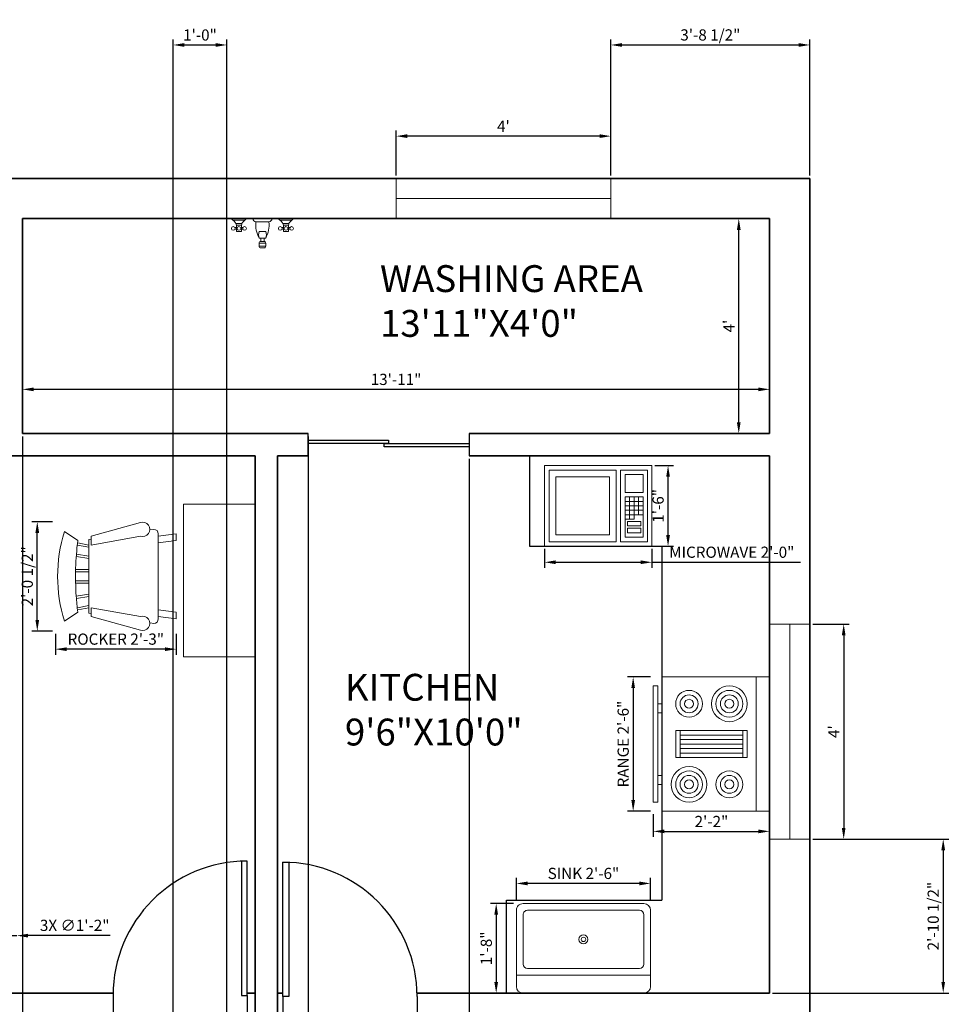
# Model space of a CAD drawing. Units: inches. Extents: x 3889 to 4254, y 3310 to 3958.
# Tile 6 of 6: x 4046 to 4254, y 3738 to 3958. Entities that reach past the tile are written whole.
import ezdxf

# ---------------------------------------------------------------- set-up
doc = ezdxf.new("R2010")
doc.units = ezdxf.units.IN
for name, color, linetype, lineweight in [('A-AREA-IDEN', 11, 'Continuous', 18), ('A-EQPM', 130, 'Continuous', 18), ('A-FLOR-CASE', 130, 'Continuous', 25), ('A-FLOR-FIXT', 130, 'Continuous', 18), ('A-WALL', 7, 'Continuous', 35), ('DIM', 81, 'Continuous', 18), ('DOOR', 1, 'Continuous', 25), ('FURNITURES', 130, 'Continuous', 18), ('WINDOW', 3, 'Continuous', 18)]:
    doc.layers.add(name, color=color, linetype=linetype, lineweight=lineweight)
doc.styles.get("Standard").update_dxf_attribs({"font": 'arial.ttf'})
doc.dimstyles.new('ISO-25', dxfattribs={"dimtxt": 2.5, "dimasz": 2.5, "dimexe": 1.25, "dimexo": 0.625, "dimtad": 1, "dimlunit": 3, "dimtxsty": 'Standard', "dimcen": 2.5, "dimadec": 0, "dimazin": 0, "dimtfac": 1, "dimtmove": 0, "dimatfit": 3, "dimfxl": 1, "dimarcsym": 0})

# ---------------------------------------------------------------- blocks, each defined once
blk = doc.blocks.new('*U4')
for p, q in [((0, 0), (0, -6)), ((40, 0), (40, -6))]:
    blk.add_line(p, q)
blk.add_lwpolyline([(0, 0), (0, 40), (1.75, 40), (1.75, 0)], close=True)
blk.add_arc((0, 0), 40, 0, 90)
blk = doc.blocks.new('*U2')
for p, q in [((0, 0), (0, -6)), ((-40, 0), (-40, -6))]:
    blk.add_line(p, q)
blk.add_lwpolyline([(0, 0), (0, 40), (-1.75, 40), (-1.75, 0)], close=True)
blk.add_arc((0, 0), 40, 90, 180)
blk = doc.blocks.new('Range-Oven - 30 in top')
for p, q in [((0, -3), (30, -3)), ((12, -6), (18, -6)), ((13, -20), (13, -6)), ((14, -6), (14, -20)), ((15, -20), (15, -6)), ((16, -6), (16, -20)), ((17, -20), (17, -6)), ((18, -20), (12, -20)), ((6, -24), (6, -25)), ((8, -25), (8, -24)), ((22, -25), (22, -24)), ((24, -24), (24, -25))]:
    blk.add_line(p, q)
for points in [[(0, -24), (0, 0), (30, 0), (30, -24)], [(12, -21), (12, -5), (18, -5), (18, -21)], [(2, -26), (2, -25), (28, -25), (28, -26)]]:
    blk.add_lwpolyline(points, close=True)
for centre, radius in [((6, -9), 4), ((6, -9), 3), ((24, -9), 3), ((6, -9), 2), ((6, -9), 1), ((24, -9), 2), ((24, -9), 1), ((6, -18), 3), ((24, -18), 4), ((24, -18), 3), ((6, -18), 2), ((6, -18), 1), ((24, -18), 2), ((24, -18), 1)]:
    blk.add_circle(centre, radius)
blk = doc.blocks.new('Sink-single - 30 in top')
blk.add_line((-15, -3.999996), (15, -3.999996))
for points in [[(-13.5, 0), (13.5, 0)], [(-15, -18.499996), (-15, -1.5)], [(15, -1.5), (15, -18.499996)], [(-13.5, -17.499996), (-13.5, -6.499996)], [(-12.5, -5.499996), (12.5, -5.499996)], [(13.5, -6.499996), (13.5, -17.499996)], [(12.5, -18.499996), (-12.5, -18.499996)], [(13.5, -19.999996), (-13.5, -19.999996)]]:
    blk.add_lwpolyline(points)
for radius in [1, 0.5]:
    blk.add_circle((0, -11.999996), radius)
for centre, radius, start, end in [((-13.5, -1.5), 1.5, 90, 180), ((13.5, -1.5), 1.5, 0, 90), ((-12.5, -6.499996), 1, 90, 180), ((12.5, -6.499996), 1, 0, 90), ((-12.5, -17.499996), 1, 180, 270), ((12.5, -17.499996), 1, 270, 0), ((-13.5, -18.499996), 1.5, 180, 270), ((13.5, -18.499996), 1.5, 270, 0)]:
    blk.add_arc(centre, radius, start, end)
blk = doc.blocks.new('Microwave')
for p, q in [((19, 7), (19, 11)), ((20, 11), (20, 7)), ((21, 7), (21, 11)), ((18, 10), (22, 10)), ((22, 9), (18, 9)), ((18, 8), (22, 8)), ((22, 7), (18, 7)), ((19, 6), (19, 7)), ((20, 7), (20, 6)), ((20, 6), (18, 6))]:
    blk.add_line(p, q)
for points in [[(0, 0), (0, 18), (24, 18), (24, 0)], [(1, 1), (1, 17), (16, 17), (16, 1)], [(2.5, 2.5), (2.5, 15.5), (14.5, 15.5), (14.5, 2.5)], [(17, 1), (17, 17), (23, 17), (23, 1)], [(18, 12), (18, 16), (22, 16), (22, 12)], [(18, 2), (18, 11), (22, 11), (22, 2)], [(18.5, 4.5), (18.5, 5.5), (21.5, 5.5), (21.5, 4.5)], [(18.5, 3), (18.5, 4), (21.5, 4), (21.5, 3)]]:
    blk.add_lwpolyline(points, close=True)
blk = doc.blocks.new('Chair - Rocking')
for p, q in [((-8, -4.5), (-10, -1.5)), ((8, -4.5), (10, -1.5)), ((-4.5, -7), (-4.96674, -4.19951)), ((-4, -7), (-4.40532, -4.16272)), ((-1.5, -4.05012), (-1.5, -7)), ((-1, -7), (-1, -4.05012)), ((1, -7), (1, -4.04655)), ((1.5, -4.05012), (1.5, -7)), ((4, -7), (4.40187, -4.18694)), ((4.5, -7), (4.96761, -4.19437)), ((-7.5, -4.5), (-7, -7)), ((-6.5, -7), (-7.02225, -4.43)), ((6.5, -7), (7, -4.4057)), ((7.5, -4.5), (7, -7)), ((-9, -7.5), (-12, -18.49999)), ((-7, -7.5), (-9, -7.5)), ((-9, -18.49999), (-7, -7.5)), ((-8.23428, -6.99939), (-8.3093, -7.47958)), ((-8.23041, -7), (8.23915, -7)), ((7, -7.5), (9, -7.5)), ((9, -18.49999), (7, -7.5)), ((8.31071, -7.48854), (8.23449, -7.00073)), ((9, -7.5), (12, -18.49999)), ((-10.36644, -20.64523), (-10.5, -21.49999)), ((10.5, -21.49999), (10.3575, -20.58798)), ((-9, -22.49999), (-9.5, -26.49999)), ((0, -22.49999), (-9.5, -22.49999)), ((-8, -26.49999), (-7.5, -22.49999)), ((0, -22.49999), (9.5, -22.49999)), ((8, -26.49999), (7.5, -22.49999)), ((9, -22.49999), (9.5, -26.49999)), ((-9.5, -26.49999), (-8, -26.49999)), ((9.5, -26.49999), (8, -26.49999))]:
    blk.add_line(p, q)
for centre, radius, start, end in [((0, -34.08333), 34.08333, 72.93847, 107.0615), ((0, -68.25004), 64.25, 93.92211, 97.15267), ((0, -68.25004), 64.25, 82.84733, 93.92211), ((-10.5, -18.99999), 1.58114, 161.5651, 18.43495), ((10.5, -18.99999), 1.58114, 161.5651, 18.43495), ((-9.5, -21.49999), 1, 180, 270), ((9.5, -21.49999), 1, 270, 0)]:
    blk.add_arc(centre, radius, start, end)
blk = doc.blocks.new('Faucet - Bathroom front')
for p, q in [((-0.5, 4.25), (0.5, 4.25)), ((0.5, 3.75), (-0.5, 3.75)), ((-0.25, 3), (-0.25, 3.5)), ((0.25, 3.5), (0.25, 3)), ((-4, 1.625), (-4.25, 1.625)), ((-3.25, 1.625), (-3, 1.625)), ((-0.5, 3), (0.5, 3)), ((0.5, 2), (-0.5, 2)), ((3.25, 1.625), (3, 1.625)), ((4, 1.625), (4.25, 1.625)), ((-5, 0), (-2.25, 0)), ((-4.5087, 0.25), (-2.7408, 0.25)), ((-4, 1.375), (-4.25, 1.375)), ((-3.1442, 0.75), (-4.0979, 0.75)), ((-3.25, 1.375), (-3, 1.375)), ((-1.5, 0), (1.5, 0)), ((-1, 0.5), (1, 0.5)), ((2.25, 0), (5, 0)), ((2.7413, 0.25), (4.5092, 0.25)), ((3.25, 1.375), (3, 1.375)), ((4.1058, 0.75), (3.1521, 0.75)), ((4, 1.375), (4.25, 1.375))]:
    blk.add_line(p, q)
for points in [[(-0.5, 3.75), (-0.5, 4.25)], [(-0.25, 4.5), (0.25, 4.5)], [(0.25, 3.5), (-0.25, 3.5)], [(0.5, 4.25), (0.5, 3.75)]]:
    blk.add_lwpolyline(points)
for points in [[(-4, 1), (-4, 2), (-3.25, 2), (-3.25, 1)], [(3.25, 1), (3.25, 2), (4, 2), (4, 1)]]:
    blk.add_lwpolyline(points, close=True)
for centre in [(-4.5, 1.5), (-3.625, 1.5), (-2.75, 1.5), (2.75, 1.5), (3.625, 1.5), (4.5, 1.5)]:
    blk.add_circle(centre, 0.2795)
for centre, radius, start, end in [((-0.2575, 4.2575), 0.2426, 88.22243, 181.7776), ((-0.2575, 3.7425), 0.2426, 178.2224, 271.7776), ((0.2575, 4.2575), 0.2426, 358.2224, 91.77757), ((0.2575, 3.7425), 0.2426, 268.2224, 1.777565), ((3, 1), 4.0311, 150.2551, 187.125), ((0.6413, 2.5), 1.246, 156.3417, 203.6583), ((-3, 1), 4.0311, 352.875, 29.74488), ((-0.6413, 2.5), 1.246, 336.3417, 23.65835), ((-5.375, 1.375), 1.4252, 285.2551, 344.7449), ((-1.875, 1.375), 1.4252, 195.2551, 254.7449), ((-0.7962, -0.2038), 0.7327, 106.1502, 163.8498), ((0.7962, -0.2038), 0.7327, 16.1502, 73.84979), ((1.875, 1.375), 1.4252, 285.2551, 344.7449), ((5.375, 1.375), 1.4252, 195.2551, 254.7449)]:
    blk.add_arc(centre, radius, start, end)
blk = doc.blocks.new('*D31')
at = {"layer": 'Defpoints', "color": 0, "transparency": 16777216}
for p in [(4206.94, 3913.11), (4213.84, 3913.11), (4213.84, 3865.11)]:
    blk.add_point(p, dxfattribs=at)
at = {"layer": 'DIM', "color": 0, "lineweight": -2, "transparency": 16777216}
for p, q in [((4213.22, 3913.11), (4205.69, 3913.11)), ((4206.94, 3867.61), (4206.94, 3910.61)), ((4213.22, 3865.11), (4205.69, 3865.11))]:
    blk.add_line(p, q, dxfattribs=at)
at = {"layer": 'DIM', "color": 0, "transparency": 16777216}
for points in [[(4206.53, 3910.61), (4207.36, 3910.61), (4206.94, 3913.11)], [(4206.53, 3867.61), (4207.36, 3867.61), (4206.94, 3865.11)]]:
    blk.add_solid(points, dxfattribs=at)
at = {"layer": 'DIM', "color": 0, "transparency": 16777216, "insert": (4205.07, 3889.11), "char_height": 2.5, "attachment_point": 5, "rotation": 90}
blk.add_mtext("4'", dxfattribs=at)
blk = doc.blocks.new('*D32')
at = {"layer": 'Defpoints', "color": 0, "transparency": 16777216}
for p in [(4046.84, 3874.98), (4046.84, 3865.11), (4213.84, 3865.11)]:
    blk.add_point(p, dxfattribs=at)
at = {"layer": 'DIM', "color": 0, "lineweight": -2, "transparency": 16777216}
for p, q in [((4046.84, 3865.73), (4046.84, 3876.23)), ((4213.84, 3865.73), (4213.84, 3876.23)), ((4211.34, 3874.98), (4049.34, 3874.98))]:
    blk.add_line(p, q, dxfattribs=at)
at = {"layer": 'DIM', "color": 0, "transparency": 16777216}
for points in [[(4049.34, 3875.39), (4049.34, 3874.56), (4046.84, 3874.98)], [(4211.34, 3875.39), (4211.34, 3874.56), (4213.84, 3874.98)]]:
    blk.add_solid(points, dxfattribs=at)
at = {"layer": 'DIM', "color": 0, "transparency": 16777216, "insert": (4130.34, 3876.88), "char_height": 2.5, "attachment_point": 5}
blk.add_mtext('13\'-11"', dxfattribs=at)
blk = doc.blocks.new('*D36')
at = {"layer": 'Defpoints', "color": 0, "transparency": 16777216}
for p in [(4130.34, 3931.54), (4130.34, 3922.11), (4178.34, 3922.11)]:
    blk.add_point(p, dxfattribs=at)
at = {"layer": 'DIM', "color": 0, "lineweight": -2, "transparency": 16777216}
for p, q in [((4130.34, 3922.73), (4130.34, 3932.79)), ((4178.34, 3922.73), (4178.34, 3932.79)), ((4175.84, 3931.54), (4132.84, 3931.54))]:
    blk.add_line(p, q, dxfattribs=at)
at = {"layer": 'DIM', "color": 0, "transparency": 16777216}
for points in [[(4132.84, 3931.96), (4132.84, 3931.13), (4130.34, 3931.54)], [(4175.84, 3931.96), (4175.84, 3931.13), (4178.34, 3931.54)]]:
    blk.add_solid(points, dxfattribs=at)
at = {"layer": 'DIM', "color": 0, "transparency": 16777216, "insert": (4154.34, 3933.42), "char_height": 2.5, "attachment_point": 5}
blk.add_mtext("4'", dxfattribs=at)
blk = doc.blocks.new('*D37')
at = {"layer": 'Defpoints', "color": 0, "transparency": 16777216}
for p in [(4222.84, 3822.52), (4222.84, 3774.52), (4230.4, 3774.52)]:
    blk.add_point(p, dxfattribs=at)
at = {"layer": 'DIM', "color": 0, "lineweight": -2, "transparency": 16777216}
for p, q in [((4223.47, 3822.52), (4231.65, 3822.52)), ((4230.4, 3820.02), (4230.4, 3777.02)), ((4223.47, 3774.52), (4231.65, 3774.52))]:
    blk.add_line(p, q, dxfattribs=at)
at = {"layer": 'DIM', "color": 0, "transparency": 16777216}
for points in [[(4229.98, 3820.02), (4230.81, 3820.02), (4230.4, 3822.52)], [(4229.98, 3777.02), (4230.81, 3777.02), (4230.4, 3774.52)]]:
    blk.add_solid(points, dxfattribs=at)
at = {"layer": 'DIM', "color": 0, "transparency": 16777216, "insert": (4228.52, 3798.52), "char_height": 2.5, "attachment_point": 5, "rotation": 90}
blk.add_mtext("4'", dxfattribs=at)
blk = doc.blocks.new('WIN-48x9')
blk.add_line((4.5, 48), (4.5, 0))
blk.add_lwpolyline([(0, 48), (9, 48), (9, 0), (0, 0)], close=True)
blk = doc.blocks.new('*D59')
at = {"layer": 'Defpoints', "color": 0, "transparency": 16777216}
for p in [(4187.84, 3810.74), (4183.34, 3780.74), (4187.84, 3780.74)]:
    blk.add_point(p, dxfattribs=at)
at = {"layer": 'DIM', "color": 0, "lineweight": -2, "transparency": 16777216}
for p, q in [((4187.22, 3810.74), (4182.09, 3810.74)), ((4183.34, 3808.24), (4183.34, 3783.24)), ((4187.22, 3780.74), (4182.09, 3780.74))]:
    blk.add_line(p, q, dxfattribs=at)
at = {"layer": 'DIM', "color": 0, "transparency": 16777216}
for points in [[(4182.93, 3808.24), (4183.76, 3808.24), (4183.34, 3810.74)], [(4182.93, 3783.24), (4183.76, 3783.24), (4183.34, 3780.74)]]:
    blk.add_solid(points, dxfattribs=at)
at = {"layer": 'DIM', "color": 0, "transparency": 16777216, "insert": (4181.43, 3795.74), "char_height": 2.5, "attachment_point": 5, "rotation": 90}
blk.add_mtext('RANGE 2\'-6"', dxfattribs=at)
blk = doc.blocks.new('*D60')
at = {"layer": 'Defpoints', "color": 0, "transparency": 16777216}
for p in [(4187.84, 3780.74), (4213.84, 3780.74), (4213.84, 3776.24)]:
    blk.add_point(p, dxfattribs=at)
at = {"layer": 'DIM', "color": 0, "lineweight": -2, "transparency": 16777216}
for p, q in [((4187.84, 3780.11), (4187.84, 3774.99)), ((4213.84, 3780.11), (4213.84, 3774.99)), ((4190.34, 3776.24), (4211.34, 3776.24))]:
    blk.add_line(p, q, dxfattribs=at)
at = {"layer": 'DIM', "color": 0, "transparency": 16777216}
for points in [[(4190.34, 3776.65), (4190.34, 3775.82), (4187.84, 3776.24)], [(4211.34, 3776.65), (4211.34, 3775.82), (4213.84, 3776.24)]]:
    blk.add_solid(points, dxfattribs=at)
at = {"layer": 'DIM', "color": 0, "transparency": 16777216, "insert": (4200.84, 3778.12), "char_height": 2.5, "attachment_point": 5}
blk.add_mtext('2\'-2"', dxfattribs=at)
blk = doc.blocks.new('*D61')
at = {"layer": 'Defpoints', "color": 0, "transparency": 16777216}
for p in [(4157.23, 3764.61), (4157.23, 3760.11), (4187.23, 3760.11)]:
    blk.add_point(p, dxfattribs=at)
at = {"layer": 'DIM', "color": 0, "lineweight": -2, "transparency": 16777216}
for p, q in [((4157.23, 3760.73), (4157.23, 3765.86)), ((4187.23, 3760.73), (4187.23, 3765.86)), ((4184.73, 3764.61), (4159.73, 3764.61))]:
    blk.add_line(p, q, dxfattribs=at)
at = {"layer": 'DIM', "color": 0, "transparency": 16777216}
for points in [[(4159.73, 3765.02), (4159.73, 3764.19), (4157.23, 3764.61)], [(4184.73, 3765.02), (4184.73, 3764.19), (4187.23, 3764.61)]]:
    blk.add_solid(points, dxfattribs=at)
at = {"layer": 'DIM', "color": 0, "transparency": 16777216, "insert": (4172.23, 3766.52), "char_height": 2.5, "attachment_point": 5}
blk.add_mtext('SINK 2\'-6"', dxfattribs=at)
blk = doc.blocks.new('*D62')
at = {"layer": 'Defpoints', "color": 0, "transparency": 16777216}
for p in [(4157.23, 3760.11), (4152.73, 3740.11), (4157.23, 3740.11)]:
    blk.add_point(p, dxfattribs=at)
at = {"layer": 'DIM', "color": 0, "lineweight": -2, "transparency": 16777216}
for p, q in [((4156.61, 3760.11), (4151.48, 3760.11)), ((4152.73, 3757.61), (4152.73, 3742.61)), ((4156.61, 3740.11), (4151.48, 3740.11))]:
    blk.add_line(p, q, dxfattribs=at)
at = {"layer": 'DIM', "color": 0, "transparency": 16777216}
for points in [[(4152.31, 3757.61), (4153.15, 3757.61), (4152.73, 3760.11)], [(4152.31, 3742.61), (4153.15, 3742.61), (4152.73, 3740.11)]]:
    blk.add_solid(points, dxfattribs=at)
at = {"layer": 'DIM', "color": 0, "transparency": 16777216, "insert": (4150.83, 3750.11), "char_height": 2.5, "attachment_point": 5, "rotation": 90}
blk.add_mtext('1\'-8"', dxfattribs=at)
blk = doc.blocks.new('*D63')
at = {"layer": 'Defpoints', "color": 0, "transparency": 16777216}
for p in [(4163.54, 3839.95), (4187.54, 3839.95), (4187.54, 3836.35)]:
    blk.add_point(p, dxfattribs=at)
at = {"layer": 'DIM', "color": 0, "lineweight": -2, "transparency": 16777216}
for p, q in [((4163.54, 3839.33), (4163.54, 3835.1)), ((4187.54, 3839.33), (4187.54, 3835.1)), ((4166.04, 3836.35), (4185.04, 3836.35)), ((4187.54, 3836.35), (4220.72, 3836.35))]:
    blk.add_line(p, q, dxfattribs=at)
at = {"layer": 'DIM', "color": 0, "transparency": 16777216}
for points in [[(4166.04, 3836.77), (4166.04, 3835.94), (4163.54, 3836.35)], [(4185.04, 3836.77), (4185.04, 3835.94), (4187.54, 3836.35)]]:
    blk.add_solid(points, dxfattribs=at)
at = {"layer": 'DIM', "color": 0, "transparency": 16777216, "insert": (4205.38, 3838.27), "char_height": 2.5, "attachment_point": 5}
blk.add_mtext('MICROWAVE 2\'-0"', dxfattribs=at)
blk = doc.blocks.new('*D64')
at = {"layer": 'Defpoints', "color": 0, "transparency": 16777216}
for p in [(4187.54, 3857.95), (4191.14, 3857.95), (4187.54, 3839.95)]:
    blk.add_point(p, dxfattribs=at)
at = {"layer": 'DIM', "color": 0, "lineweight": -2, "transparency": 16777216}
for p, q in [((4188.17, 3857.95), (4192.39, 3857.95)), ((4191.14, 3842.45), (4191.14, 3855.45)), ((4188.17, 3839.95), (4192.39, 3839.95))]:
    blk.add_line(p, q, dxfattribs=at)
at = {"layer": 'DIM', "color": 0, "transparency": 16777216}
for points in [[(4190.72, 3855.45), (4191.56, 3855.45), (4191.14, 3857.95)], [(4190.72, 3842.45), (4191.56, 3842.45), (4191.14, 3839.95)]]:
    blk.add_solid(points, dxfattribs=at)
at = {"layer": 'DIM', "color": 0, "transparency": 16777216, "insert": (4189.24, 3848.95), "char_height": 2.5, "attachment_point": 5, "rotation": 90}
blk.add_mtext('1\'-6"', dxfattribs=at)
blk = doc.blocks.new('*D65')
at = {"layer": 'Defpoints', "color": 0, "transparency": 16777216}
for p in [(4054.21, 3820.99), (4081.21, 3820.99), (4054.21, 3816.94)]:
    blk.add_point(p, dxfattribs=at)
at = {"layer": 'DIM', "color": 0, "lineweight": -2, "transparency": 16777216}
for p, q in [((4054.21, 3820.36), (4054.21, 3815.69)), ((4081.21, 3820.36), (4081.21, 3815.69)), ((4078.71, 3816.94), (4056.71, 3816.94))]:
    blk.add_line(p, q, dxfattribs=at)
at = {"layer": 'DIM', "color": 0, "transparency": 16777216}
for points in [[(4056.71, 3817.35), (4056.71, 3816.52), (4054.21, 3816.94)], [(4078.71, 3817.35), (4078.71, 3816.52), (4081.21, 3816.94)]]:
    blk.add_solid(points, dxfattribs=at)
at = {"layer": 'DIM', "color": 0, "transparency": 16777216, "insert": (4067.71, 3818.86), "char_height": 2.5, "attachment_point": 5}
blk.add_mtext('ROCKER 2\'-3"', dxfattribs=at)
blk = doc.blocks.new('*D66')
at = {"layer": 'Defpoints', "color": 0, "transparency": 16777216}
for p in [(4050.16, 3845.42), (4054.21, 3845.42), (4054.21, 3820.99)]:
    blk.add_point(p, dxfattribs=at)
at = {"layer": 'DIM', "color": 0, "lineweight": -2, "transparency": 16777216}
for p, q in [((4053.58, 3845.42), (4048.91, 3845.42)), ((4050.16, 3823.49), (4050.16, 3842.92)), ((4053.58, 3820.99), (4048.91, 3820.99))]:
    blk.add_line(p, q, dxfattribs=at)
at = {"layer": 'DIM', "color": 0, "transparency": 16777216}
for points in [[(4049.74, 3842.92), (4050.57, 3842.92), (4050.16, 3845.42)], [(4049.74, 3823.49), (4050.57, 3823.49), (4050.16, 3820.99)]]:
    blk.add_solid(points, dxfattribs=at)
at = {"layer": 'DIM', "color": 0, "transparency": 16777216, "insert": (4048.24, 3833.21), "char_height": 2.5, "attachment_point": 5, "rotation": 90}
blk.add_mtext('2\'-0 1/2"', dxfattribs=at)
blk = doc.blocks.new('*D71')
at = {"layer": 'Defpoints', "color": 0, "transparency": 16777216}
for p in [(4092.52, 3951.91), (4080.52, 3351.11), (4092.52, 3351.11)]:
    blk.add_point(p, dxfattribs=at)
at = {"layer": 'DIM', "color": 0, "lineweight": -2, "transparency": 16777216}
for p, q in [((4080.52, 3351.73), (4080.52, 3953.16)), ((4092.52, 3351.73), (4092.52, 3953.16)), ((4083.02, 3951.91), (4090.02, 3951.91))]:
    blk.add_line(p, q, dxfattribs=at)
at = {"layer": 'DIM', "color": 0, "transparency": 16777216}
for points in [[(4083.02, 3952.32), (4083.02, 3951.49), (4080.52, 3951.91)], [(4090.02, 3952.32), (4090.02, 3951.49), (4092.52, 3951.91)]]:
    blk.add_solid(points, dxfattribs=at)
at = {"layer": 'DIM', "color": 0, "transparency": 16777216, "insert": (4086.52, 3953.81), "char_height": 2.5, "attachment_point": 5}
blk.add_mtext('1\'-0"', dxfattribs=at)
blk = doc.blocks.new('*D76')
at = {"layer": 'Defpoints', "color": 0, "transparency": 16777216}
for p in [(4222.84, 3951.91), (4178.34, 3922.11), (4222.84, 3922.11)]:
    blk.add_point(p, dxfattribs=at)
at = {"layer": 'DIM', "color": 0, "lineweight": -2, "transparency": 16777216}
for p, q in [((4178.34, 3922.73), (4178.34, 3953.16)), ((4222.84, 3922.73), (4222.84, 3953.16)), ((4180.84, 3951.91), (4220.34, 3951.91))]:
    blk.add_line(p, q, dxfattribs=at)
at = {"layer": 'DIM', "color": 0, "transparency": 16777216}
for points in [[(4180.84, 3952.32), (4180.84, 3951.49), (4178.34, 3951.91)], [(4220.34, 3952.32), (4220.34, 3951.49), (4222.84, 3951.91)]]:
    blk.add_solid(points, dxfattribs=at)
at = {"layer": 'DIM', "color": 0, "transparency": 16777216, "insert": (4200.59, 3953.83), "char_height": 2.5, "attachment_point": 5}
blk.add_mtext('3\'-8 1/2"', dxfattribs=at)
blk = doc.blocks.new('*D77')
at = {"layer": 'Defpoints', "color": 0, "transparency": 16777216}
for p in [(4222.84, 3774.52), (4213.84, 3740.11), (4252.64, 3740.11)]:
    blk.add_point(p, dxfattribs=at)
at = {"layer": 'DIM', "color": 0, "lineweight": -2, "transparency": 16777216}
for p, q in [((4223.47, 3774.52), (4253.89, 3774.52)), ((4252.64, 3772.02), (4252.64, 3742.61)), ((4214.47, 3740.11), (4253.89, 3740.11))]:
    blk.add_line(p, q, dxfattribs=at)
at = {"layer": 'DIM', "color": 0, "transparency": 16777216}
for points in [[(4252.23, 3772.02), (4253.06, 3772.02), (4252.64, 3774.52)], [(4252.23, 3742.61), (4253.06, 3742.61), (4252.64, 3740.11)]]:
    blk.add_solid(points, dxfattribs=at)
at = {"layer": 'DIM', "color": 0, "transparency": 16777216, "insert": (4250.73, 3757.31), "char_height": 2.5, "attachment_point": 5, "rotation": 90}
blk.add_mtext('2\'-10 1/2"', dxfattribs=at)
blk = doc.blocks.new('*D85')
at = {"layer": 'Defpoints', "color": 0, "transparency": 16777216}
for p in [(4110.69, 3860.11), (4146.69, 3860.11), (4146.69, 3312.31)]:
    blk.add_point(p, dxfattribs=at)
at = {"layer": 'DIM', "color": 0, "lineweight": -2, "transparency": 16777216}
for p, q in [((4110.69, 3859.48), (4110.69, 3311.06)), ((4146.69, 3859.48), (4146.69, 3311.06)), ((4113.19, 3312.31), (4144.19, 3312.31))]:
    blk.add_line(p, q, dxfattribs=at)
at = {"layer": 'DIM', "color": 0, "transparency": 16777216}
for points in [[(4113.19, 3312.72), (4113.19, 3311.89), (4110.69, 3312.31)], [(4144.19, 3312.72), (4144.19, 3311.89), (4146.69, 3312.31)]]:
    blk.add_solid(points, dxfattribs=at)
at = {"layer": 'DIM', "color": 0, "transparency": 16777216, "insert": (4128.69, 3314.21), "char_height": 2.5, "attachment_point": 5}
blk.add_mtext('3\'-0"', dxfattribs=at)
blk = doc.blocks.new('*D86')
at = {"layer": 'Defpoints', "color": 0, "transparency": 16777216}
for p in [(4046.84, 3865.11), (4110.69, 3865.11), (4110.69, 3312.31)]:
    blk.add_point(p, dxfattribs=at)
at = {"layer": 'DIM', "color": 0, "lineweight": -2, "transparency": 16777216}
for p, q in [((4046.84, 3864.48), (4046.84, 3311.06)), ((4110.69, 3864.48), (4110.69, 3311.06)), ((4049.34, 3312.31), (4108.19, 3312.31))]:
    blk.add_line(p, q, dxfattribs=at)
at = {"layer": 'DIM', "color": 0, "transparency": 16777216}
for points in [[(4049.34, 3312.72), (4049.34, 3311.89), (4046.84, 3312.31)], [(4108.19, 3312.72), (4108.19, 3311.89), (4110.69, 3312.31)]]:
    blk.add_solid(points, dxfattribs=at)
at = {"layer": 'DIM', "color": 0, "transparency": 16777216, "insert": (4078.77, 3314.2), "char_height": 2.5, "attachment_point": 5}
blk.add_mtext('5\'-4"', dxfattribs=at)
blk = doc.blocks.new('*D95')
at = {"layer": 'Defpoints', "color": 0, "transparency": 16777216}
for p in [(4046.84, 3865.11), (4098.84, 3860.11), (4098.84, 3312.31)]:
    blk.add_point(p, dxfattribs=at)
at = {"layer": 'DIM', "color": 0, "lineweight": -2, "transparency": 16777216}
for p, q in [((4046.84, 3864.48), (4046.84, 3311.06)), ((4098.84, 3859.48), (4098.84, 3311.06)), ((4049.34, 3312.31), (4096.34, 3312.31))]:
    blk.add_line(p, q, dxfattribs=at)
at = {"layer": 'DIM', "color": 0, "transparency": 16777216}
for points in [[(4049.34, 3312.72), (4049.34, 3311.89), (4046.84, 3312.31)], [(4096.34, 3312.72), (4096.34, 3311.89), (4098.84, 3312.31)]]:
    blk.add_solid(points, dxfattribs=at)
at = {"layer": 'DIM', "color": 0, "transparency": 16777216, "insert": (4072.84, 3314.18), "char_height": 2.5, "attachment_point": 5}
blk.add_mtext('4\'-4"', dxfattribs=at)
blk = doc.blocks.new('*D98')
at = {"layer": 'Defpoints', "color": 0, "transparency": 16777216}
for p in [(4031.6, 3752.95), (4045.6, 3752.95)]:
    blk.add_point(p, dxfattribs=at)
at = {"layer": 'DIM', "color": 0, "lineweight": -2, "transparency": 16777216}
for p, q in [((4029.1, 3752.94), (4026.6, 3752.94)), ((4031.6, 3752.95), (4045.6, 3752.95)), ((4066.45, 3752.95), (4048.1, 3752.95))]:
    blk.add_line(p, q, dxfattribs=at)
at = {"layer": 'DIM', "color": 0, "transparency": 16777216}
for points in [[(4029.1, 3753.36), (4029.1, 3752.53), (4031.6, 3752.95)], [(4048.1, 3753.37), (4048.1, 3752.53), (4045.6, 3752.95)]]:
    blk.add_solid(points, dxfattribs=at)
at = {"layer": 'DIM', "color": 0, "transparency": 16777216, "insert": (4058.52, 3754.92), "char_height": 2.5, "attachment_point": 5, "rotation": 0.0136}
blk.add_mtext('3X ∅1\'-2"', dxfattribs=at)

msp = doc.modelspace()

# ---------------------------------------------------------------- linework, layer by layer
at = {"layer": 'A-FLOR-CASE'}
for points in [[(4213.843, 3839.953), (4213.843, 3860.107), (4160.186, 3860.107), (4160.186, 3839.953), (4189.754, 3839.953)], [(4189.754, 3740.107), (4213.843, 3740.107), (4213.843, 3860.107), (4189.754, 3860.107)], [(4189.754, 3839.953), (4189.754, 3760.875)], [(4213.843, 3760.875), (4213.843, 3740.107), (4155.029, 3740.107), (4155.029, 3760.875), (4189.754, 3760.875)]]:
    msp.add_lwpolyline(points, dxfattribs=at)
at = {"layer": 'A-WALL'}
for p, q in [((3924.843, 3922.107), (4222.843, 3922.107)), ((4222.843, 3342.107), (4222.843, 3922.107)), ((4046.843, 3865.107), (4046.843, 3913.107)), ((4046.843, 3913.107), (4213.843, 3913.107)), ((4213.843, 3865.107), (4213.843, 3913.107)), ((4046.843, 3865.107), (4110.69, 3865.107)), ((4146.69, 3865.107), (4213.843, 3865.107)), ((3967.546, 3860.107), (4098.843, 3860.107)), ((4098.843, 3735.107), (4098.843, 3860.107)), ((4103.843, 3735.107), (4103.843, 3860.107)), ((4103.843, 3860.107), (4110.69, 3860.107)), ((4146.69, 3860.107), (4213.843, 3860.107)), ((4213.843, 3740.107), (4213.843, 3860.107)), ((3933.843, 3740.107), (4067.084, 3740.107)), ((4097.08, 3740.107), (4098.843, 3740.107)), ((4103.843, 3740.107), (4105.044, 3740.107)), ((4135.034, 3740.107), (4213.843, 3740.107))]:
    msp.add_line(p, q, dxfattribs=at)
at = {"layer": 'DOOR'}
for points in [[(4110.69, 3860.107), (4110.69, 3865.107)], [(4146.69, 3865.107), (4146.69, 3860.107)]]:
    msp.add_lwpolyline(points, dxfattribs=at)
for points in [[(4110.69, 3863.594), (4128.69, 3863.594), (4128.69, 3862.883), (4110.69, 3862.883)], [(4127.672, 3862.883), (4146.69, 3862.883), (4146.69, 3862.171), (4127.672, 3862.171)]]:
    msp.add_lwpolyline(points, close=True, dxfattribs=at)
at = {"layer": 'FURNITURES'}
msp.add_lwpolyline([(4098.843, 3849.36), (4082.858, 3849.36), (4082.858, 3815.234), (4098.843, 3815.234)], close=True, dxfattribs=at)

# ---------------------------------------------------------------- block references
at = {"layer": 'A-EQPM'}
msp.add_blockref('Microwave', (4163.541, 3839.953), dxfattribs=at)
at = {"layer": 'A-EQPM', "rotation": 270}
msp.add_blockref('Range-Oven - 30 in top', (4213.843, 3810.736), dxfattribs=at)
at = {"layer": 'A-FLOR-FIXT', "xscale": 1.450441564443806, "yscale": 1.450441564443806, "zscale": 1.450441564443806, "rotation": 180}
msp.add_blockref('Faucet - Bathroom front', (4100.478, 3913.107), dxfattribs=at)
at = {"layer": 'A-FLOR-FIXT', "rotation": 180}
msp.add_blockref('Sink-single - 30 in top', (4172.231, 3740.107), dxfattribs=at)
at = {"layer": 'DOOR', "xscale": 0.75, "yscale": 0.75, "zscale": 0.75}
for name, p in [('*U2', (4097.08, 3739.607)), ('*U4', (4105.044, 3739.339))]:
    msp.add_blockref(name, p, dxfattribs=at)
at = {"layer": 'FURNITURES', "rotation": 90}
msp.add_blockref('Chair - Rocking', (4054.706, 3833.205), dxfattribs=at)
at = {"layer": 'WINDOW', "rotation": 270.0000000000007}
msp.add_blockref('WIN-48x9', (4130.343, 3922.107), dxfattribs=at)
at = {"layer": 'WINDOW'}
msp.add_blockref('WIN-48x9', (4213.843, 3774.518), dxfattribs=at)

# ---------------------------------------------------------------- texts
at = {"layer": 'A-AREA-IDEN', "char_height": 6, "attachment_point": 1}
for s, insert in [('WASHING AREA\\P13\'11"X4\'0"', (4126.753, 3902.712)), ('KITCHEN\\P9\'6"X10\'0"', (4118.918, 3811.428))]:
    msp.add_mtext_dynamic_manual_height_columns(s, width=76.4548, gutter_width=12.5, heights=[0], dxfattribs=dict(at, insert=insert))

# ---------------------------------------------------------------- dimensions: what is measured, and where the dimension line sits
at = {"layer": 'DIM'}
for base, p1, p2, override, picture, middle in [((4222.843, 3951.907), (4178.343, 3922.107), (4222.843, 3922.107), {"dimdec": 1, "dimlfac": 1, "dimrnd": 0, "dimzin": 1, "dimdsep": 46, "dimlunit": 4, "dimfrac": 2}, '*D76', (4200.593, 3953.826)), ((4092.518, 3951.907), (4080.518, 3351.107), (4092.518, 3351.107), {"dimdec": 1, "dimlfac": 1, "dimrnd": 0, "dimzin": 1, "dimdsep": 46, "dimlunit": 4, "dimfrac": 2}, '*D71', (4086.518, 3953.808)), ((4130.343, 3931.544), (4178.343, 3922.107), (4130.343, 3922.107), {"dimclrd": 0, "dimclre": 0, "dimclrt": 0}, '*D36', (4154.343, 3933.419)), ((4046.843, 3874.977), (4213.843, 3865.107), (4046.843, 3865.107), {"dimclrd": 0, "dimclre": 0, "dimclrt": 0}, '*D32', (4130.343, 3876.879)), ((4110.69, 3312.307), (4046.843, 3865.107), (4110.69, 3865.107), {"dimdec": 1, "dimlfac": 1, "dimrnd": 0, "dimzin": 1, "dimdsep": 46, "dimlunit": 4, "dimfrac": 2}, '*D86', (4078.766, 3314.203)), ((4098.843, 3312.307), (4046.843, 3865.107), (4098.843, 3860.107), {"dimdec": 1, "dimlfac": 1, "dimrnd": 0, "dimzin": 1, "dimdsep": 46, "dimlunit": 4, "dimfrac": 2}, '*D95', (4072.843, 3314.182)), ((4146.69, 3312.307), (4110.69, 3860.107), (4146.69, 3860.107), {"dimdec": 1, "dimlfac": 1, "dimrnd": 0, "dimzin": 1, "dimdsep": 46, "dimlunit": 4, "dimfrac": 2}, '*D85', (4128.69, 3314.209)), ((4213.843, 3776.236), (4187.843, 3780.736), (4213.843, 3780.736), {"dimdec": 1, "dimlfac": 1, "dimrnd": 0, "dimzin": 1, "dimdsep": 46, "dimlunit": 4, "dimfrac": 2}, '*D60', (4200.843, 3778.116))]:
    dim = msp.add_linear_dim(base=base, p1=p1, p2=p2, dimstyle='ISO-25', override=override, dxfattribs=at)
    dim.commit()
    dim.dimension.update_dxf_attribs({"geometry": picture, "text_midpoint": middle})
for base, p1, p2, angle, override, picture, middle in [((4206.943, 3913.107), (4213.843, 3865.107), (4213.843, 3913.107), 90, {"dimclrd": 0, "dimclre": 0, "dimclrt": 0}, '*D31', (4205.068, 3889.107)), ((4191.141, 3857.953), (4187.541, 3839.953), (4187.541, 3857.953), 90, {"dimdec": 1, "dimlfac": 1, "dimrnd": 0, "dimzin": 1, "dimdsep": 46, "dimlunit": 4, "dimfrac": 2}, '*D64', (4189.239, 3848.953)), ((4050.156, 3845.423), (4054.206, 3820.988), (4054.206, 3845.423), 90, {"dimdec": 1, "dimlfac": 1, "dimrnd": 0, "dimzin": 1, "dimdsep": 46, "dimlunit": 4, "dimfrac": 2}, '*D66', (4048.239, 3833.205)), ((4230.395, 3774.518), (4222.843, 3822.518), (4222.843, 3774.518), 90, {"dimclrd": 0, "dimclre": 0, "dimclrt": 0}, '*D37', (4228.52, 3798.518)), ((4252.643, 3740.107), (4222.843, 3774.518), (4213.843, 3740.107), 90, {"dimdec": 1, "dimlfac": 1, "dimrnd": 0, "dimzin": 1, "dimdsep": 46, "dimlunit": 4, "dimfrac": 2}, '*D77', (4250.725, 3757.312)), ((4152.731, 3740.107), (4157.231, 3760.107), (4157.231, 3740.107), 270, {"dimdec": 1, "dimlfac": 1, "dimrnd": 0, "dimzin": 1, "dimdsep": 46, "dimlunit": 4, "dimfrac": 2}, '*D62', (4150.83, 3750.107))]:
    dim = msp.add_linear_dim(base=base, p1=p1, p2=p2, angle=angle, dimstyle='ISO-25', override=override, dxfattribs=at)
    dim.commit()
    dim.dimension.update_dxf_attribs({"geometry": picture, "text_midpoint": middle})
dim = msp.add_linear_dim(base=(4187.541, 3836.353), p1=(4163.541, 3839.953), p2=(4187.541, 3839.953), text='MICROWAVE <>', dimstyle='ISO-25', override={"dimdec": 1, "dimlfac": 1, "dimrnd": 0, "dimzin": 1, "dimdsep": 46, "dimlunit": 4, "dimfrac": 2}, dxfattribs=at)
dim.commit()
dim.dimension.update_dxf_attribs({"geometry": '*D63', "text_midpoint": (4205.379, 3838.272)})
for base, p1, p2, angle, text, picture, middle in [((4054.206, 3816.938), (4081.206, 3820.988), (4054.206, 3820.988), 180, 'ROCKER <>', '*D65', (4067.706, 3818.857)), ((4183.343, 3780.736), (4187.843, 3810.736), (4187.843, 3780.736), 270, 'RANGE <>', '*D59', (4181.425, 3795.736)), ((4157.231, 3764.607), (4187.231, 3760.107), (4157.231, 3760.107), 180, 'SINK <>', '*D61', (4172.231, 3766.525))]:
    dim = msp.add_linear_dim(base=base, p1=p1, p2=p2, angle=angle, text=text, dimstyle='ISO-25', override={"dimdec": 1, "dimlfac": 1, "dimrnd": 0, "dimzin": 1, "dimdsep": 46, "dimlunit": 4, "dimfrac": 2}, dxfattribs=at)
    dim.commit()
    dim.dimension.update_dxf_attribs({"geometry": picture, "text_midpoint": middle})
dim = msp.add_diameter_dim_2p(p1=(4031.597, 3752.945), p2=(4045.597, 3752.948), text='3X <>', dimstyle='ISO-25', override={"dimdec": 1, "dimlfac": 1, "dimrnd": 0, "dimzin": 1, "dimdsep": 46, "dimlunit": 4, "dimfrac": 2}, dxfattribs=at)
dim.commit()
dim.dimension.update_dxf_attribs({"geometry": '*D98', "text_midpoint": (4058.524, 3752.951), "dimtype": 163})

doc.saveas('drawing.dxf')
